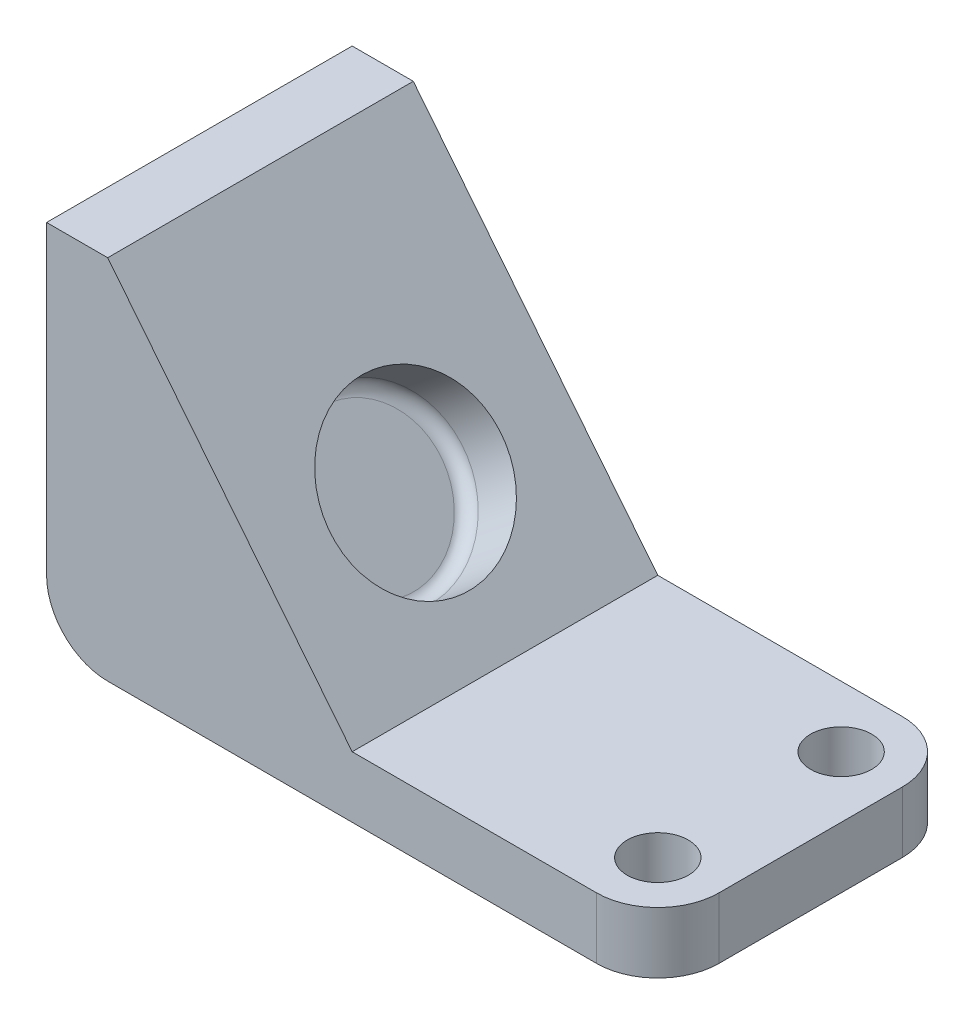
ISO-10303-21;
HEADER;
FILE_DESCRIPTION(('STEP AP214'),'2;1');
FILE_NAME('part.step','',(''),(''),'','','');
FILE_SCHEMA(('AUTOMOTIVE_DESIGN { 1 0 10303 214 1 1 1 1 }'));
ENDSEC;
DATA;
#1=APPLICATION_CONTEXT('core data for automotive mechanical design processes');
#2=APPLICATION_PROTOCOL_DEFINITION('international standard','automotive_design',2000,#1);
#3=PRODUCT_CONTEXT('',#1,'mechanical');
#4=PRODUCT('Part','Part','',(#3));
#5=PRODUCT_RELATED_PRODUCT_CATEGORY('part','',(#4));
#6=PRODUCT_DEFINITION_FORMATION('','',#4);
#7=PRODUCT_DEFINITION_CONTEXT('part definition',#1,'design');
#8=PRODUCT_DEFINITION('design','',#6,#7);
#9=PRODUCT_DEFINITION_SHAPE('','',#8);
#10=(LENGTH_UNIT() NAMED_UNIT(*) SI_UNIT(.MILLI.,.METRE.));
#11=(NAMED_UNIT(*) PLANE_ANGLE_UNIT() SI_UNIT($,.RADIAN.));
#12=(NAMED_UNIT(*) SI_UNIT($,.STERADIAN.) SOLID_ANGLE_UNIT());
#13=UNCERTAINTY_MEASURE_WITH_UNIT(LENGTH_MEASURE(1.E-05),#10,'distance_accuracy_value','');
#14=(GEOMETRIC_REPRESENTATION_CONTEXT(3) GLOBAL_UNCERTAINTY_ASSIGNED_CONTEXT((#13)) GLOBAL_UNIT_ASSIGNED_CONTEXT((#10,
#11,#12)) REPRESENTATION_CONTEXT('',''));
#15=CARTESIAN_POINT('',(0.,0.,0.));
#16=DIRECTION('',(0.,0.,1.));
#17=DIRECTION('',(1.,0.,0.));
#18=AXIS2_PLACEMENT_3D('',#15,#16,#17);
#19=CARTESIAN_POINT('',(0.,6.,2.5));
#20=DIRECTION('',(0.,-1.,0.));
#21=DIRECTION('',(0.,0.,-1.));
#22=AXIS2_PLACEMENT_3D('',#19,#20,#21);
#23=PLANE('',#22);
#24=DIRECTION('',(-1.,0.,0.));
#25=VECTOR('',#24,1.);
#26=CARTESIAN_POINT('',(0.,6.,-2.5));
#27=LINE('',#26,#25);
#28=CARTESIAN_POINT('',(1.,6.,-2.5));
#29=VERTEX_POINT('',#28);
#30=CARTESIAN_POINT('',(0.,6.,-2.5));
#31=VERTEX_POINT('',#30);
#32=EDGE_CURVE('E140',#29,#31,#27,.T.);
#33=ORIENTED_EDGE('',*,*,#32,.T.);
#34=DIRECTION('',(0.,0.,-1.));
#35=VECTOR('',#34,1.);
#36=CARTESIAN_POINT('',(0.,6.,2.5));
#37=LINE('',#36,#35);
#38=CARTESIAN_POINT('',(0.,6.,2.5));
#39=VERTEX_POINT('',#38);
#40=EDGE_CURVE('E120',#39,#31,#37,.T.);
#41=ORIENTED_EDGE('',*,*,#40,.F.);
#42=DIRECTION('',(-1.,0.,0.));
#43=VECTOR('',#42,1.);
#44=CARTESIAN_POINT('',(0.,6.,2.5));
#45=LINE('',#44,#43);
#46=CARTESIAN_POINT('',(1.,6.,2.5));
#47=VERTEX_POINT('',#46);
#48=EDGE_CURVE('E122',#47,#39,#45,.T.);
#49=ORIENTED_EDGE('',*,*,#48,.F.);
#50=DIRECTION('',(0.,0.,-1.));
#51=VECTOR('',#50,1.);
#52=CARTESIAN_POINT('',(1.,6.,2.5));
#53=LINE('',#52,#51);
#54=EDGE_CURVE('E208',#47,#29,#53,.T.);
#55=ORIENTED_EDGE('',*,*,#54,.T.);
#56=EDGE_LOOP('',(#33,#41,#49,#55));
#57=FACE_BOUND('',#56,.T.);
#58=ADVANCED_FACE('F39',(#57),#23,.F.);
#59=CARTESIAN_POINT('',(0.,1.00000000000001,2.5));
#60=DIRECTION('',(1.,0.,0.));
#61=DIRECTION('',(0.,0.,-1.));
#62=AXIS2_PLACEMENT_3D('',#59,#60,#61);
#63=PLANE('',#62);
#64=DIRECTION('',(0.,-1.,0.));
#65=VECTOR('',#64,1.);
#66=CARTESIAN_POINT('',(0.,1.00000000000001,-2.5));
#67=LINE('',#66,#65);
#68=CARTESIAN_POINT('',(0.,1.00000000000001,-2.5));
#69=VERTEX_POINT('',#68);
#70=EDGE_CURVE('E209',#31,#69,#67,.T.);
#71=ORIENTED_EDGE('',*,*,#70,.T.);
#72=DIRECTION('',(0.,0.,-1.));
#73=VECTOR('',#72,1.);
#74=CARTESIAN_POINT('',(0.,1.00000000000001,2.5));
#75=LINE('',#74,#73);
#76=CARTESIAN_POINT('',(0.,1.00000000000001,2.5));
#77=VERTEX_POINT('',#76);
#78=EDGE_CURVE('E119',#77,#69,#75,.T.);
#79=ORIENTED_EDGE('',*,*,#78,.F.);
#80=DIRECTION('',(0.,-1.,0.));
#81=VECTOR('',#80,1.);
#82=CARTESIAN_POINT('',(0.,1.00000000000001,2.5));
#83=LINE('',#82,#81);
#84=EDGE_CURVE('E114',#39,#77,#83,.T.);
#85=ORIENTED_EDGE('',*,*,#84,.F.);
#86=ORIENTED_EDGE('',*,*,#40,.T.);
#87=EDGE_LOOP('',(#71,#79,#85,#86));
#88=FACE_BOUND('',#87,.T.);
#89=ADVANCED_FACE('F113',(#88),#63,.F.);
#90=CARTESIAN_POINT('',(1.,1.,2.5));
#91=DIRECTION('',(0.,0.,-1.));
#92=DIRECTION('',(-1.,0.,0.));
#93=AXIS2_PLACEMENT_3D('',#90,#91,#92);
#94=CYLINDRICAL_SURFACE('',#93,1.);
#95=CARTESIAN_POINT('',(1.,1.,-2.5));
#96=DIRECTION('',(0.,0.,1.));
#97=DIRECTION('',(1.,0.,0.));
#98=AXIS2_PLACEMENT_3D('',#95,#96,#97);
#99=CIRCLE('',#98,1.);
#100=CARTESIAN_POINT('',(1.00000000000001,0.,-2.5));
#101=VERTEX_POINT('',#100);
#102=EDGE_CURVE('E213',#69,#101,#99,.T.);
#103=ORIENTED_EDGE('',*,*,#102,.T.);
#104=DIRECTION('',(0.,0.,-1.));
#105=VECTOR('',#104,1.);
#106=CARTESIAN_POINT('',(1.00000000000001,0.,2.5));
#107=LINE('',#106,#105);
#108=CARTESIAN_POINT('',(1.00000000000001,0.,2.5));
#109=VERTEX_POINT('',#108);
#110=EDGE_CURVE('E141',#109,#101,#107,.T.);
#111=ORIENTED_EDGE('',*,*,#110,.F.);
#112=CARTESIAN_POINT('',(1.,1.,2.5));
#113=DIRECTION('',(0.,0.,1.));
#114=DIRECTION('',(1.,0.,0.));
#115=AXIS2_PLACEMENT_3D('',#112,#113,#114);
#116=CIRCLE('',#115,1.);
#117=EDGE_CURVE('E121',#77,#109,#116,.T.);
#118=ORIENTED_EDGE('',*,*,#117,.F.);
#119=ORIENTED_EDGE('',*,*,#78,.T.);
#120=EDGE_LOOP('',(#103,#111,#118,#119));
#121=FACE_BOUND('',#120,.T.);
#122=ADVANCED_FACE('F176',(#121),#94,.T.);
#123=CARTESIAN_POINT('',(10.,0.,2.5));
#124=DIRECTION('',(0.,1.,0.));
#125=DIRECTION('',(-1.,0.,0.));
#126=AXIS2_PLACEMENT_3D('',#123,#124,#125);
#127=PLANE('',#126);
#128=CARTESIAN_POINT('',(9.,0.,1.5));
#129=DIRECTION('',(0.,1.,0.));
#130=DIRECTION('',(0.,0.,1.));
#131=AXIS2_PLACEMENT_3D('',#128,#129,#130);
#132=CIRCLE('',#131,0.500000000000001);
#133=CARTESIAN_POINT('',(9.,0.,2.));
#134=VERTEX_POINT('',#133);
#135=EDGE_CURVE('E275',#134,#134,#132,.T.);
#136=ORIENTED_EDGE('',*,*,#135,.T.);
#137=EDGE_LOOP('',(#136));
#138=FACE_BOUND('',#137,.T.);
#139=CARTESIAN_POINT('',(9.,0.,-1.5));
#140=DIRECTION('',(0.,1.,0.));
#141=DIRECTION('',(0.,0.,1.));
#142=AXIS2_PLACEMENT_3D('',#139,#140,#141);
#143=CIRCLE('',#142,0.500000000000001);
#144=CARTESIAN_POINT('',(9.,0.,-0.999999999999999));
#145=VERTEX_POINT('',#144);
#146=EDGE_CURVE('E262',#145,#145,#143,.T.);
#147=ORIENTED_EDGE('',*,*,#146,.T.);
#148=EDGE_LOOP('',(#147));
#149=FACE_BOUND('',#148,.T.);
#150=DIRECTION('',(0.,0.,-1.));
#151=VECTOR('',#150,1.);
#152=CARTESIAN_POINT('',(10.,0.,2.5));
#153=LINE('',#152,#151);
#154=CARTESIAN_POINT('',(10.,0.,1.5));
#155=VERTEX_POINT('',#154);
#156=CARTESIAN_POINT('',(10.,0.,-1.5));
#157=VERTEX_POINT('',#156);
#158=EDGE_CURVE('E200',#155,#157,#153,.T.);
#159=ORIENTED_EDGE('',*,*,#158,.F.);
#160=CARTESIAN_POINT('',(9.,0.,1.5));
#161=DIRECTION('',(0.,1.,0.));
#162=DIRECTION('',(-1.,0.,0.));
#163=AXIS2_PLACEMENT_3D('',#160,#161,#162);
#164=CIRCLE('',#163,1.);
#165=CARTESIAN_POINT('',(9.,0.,2.5));
#166=VERTEX_POINT('',#165);
#167=EDGE_CURVE('E156',#155,#166,#164,.F.);
#168=ORIENTED_EDGE('',*,*,#167,.T.);
#169=DIRECTION('',(1.,0.,0.));
#170=VECTOR('',#169,1.);
#171=CARTESIAN_POINT('',(10.,0.,2.5));
#172=LINE('',#171,#170);
#173=EDGE_CURVE('E196',#109,#166,#172,.T.);
#174=ORIENTED_EDGE('',*,*,#173,.F.);
#175=ORIENTED_EDGE('',*,*,#110,.T.);
#176=DIRECTION('',(1.,0.,0.));
#177=VECTOR('',#176,1.);
#178=CARTESIAN_POINT('',(10.,0.,-2.5));
#179=LINE('',#178,#177);
#180=CARTESIAN_POINT('',(9.,0.,-2.5));
#181=VERTEX_POINT('',#180);
#182=EDGE_CURVE('E214',#101,#181,#179,.T.);
#183=ORIENTED_EDGE('',*,*,#182,.T.);
#184=CARTESIAN_POINT('',(9.,0.,-1.5));
#185=DIRECTION('',(0.,1.,0.));
#186=DIRECTION('',(-1.,0.,0.));
#187=AXIS2_PLACEMENT_3D('',#184,#185,#186);
#188=CIRCLE('',#187,1.);
#189=EDGE_CURVE('E61',#181,#157,#188,.F.);
#190=ORIENTED_EDGE('',*,*,#189,.T.);
#191=EDGE_LOOP('',(#159,#168,#174,#175,#183,#190));
#192=FACE_BOUND('',#191,.T.);
#193=ADVANCED_FACE('F198',(#138,#149,#192),#127,.F.);
#194=CARTESIAN_POINT('',(10.,0.999999999999999,2.5));
#195=DIRECTION('',(-1.,0.,0.));
#196=DIRECTION('',(0.,0.,1.));
#197=AXIS2_PLACEMENT_3D('',#194,#195,#196);
#198=PLANE('',#197);
#199=DIRECTION('',(0.,0.,-1.));
#200=VECTOR('',#199,1.);
#201=CARTESIAN_POINT('',(10.,0.999999999999999,2.5));
#202=LINE('',#201,#200);
#203=CARTESIAN_POINT('',(10.,0.999999999999999,1.5));
#204=VERTEX_POINT('',#203);
#205=CARTESIAN_POINT('',(10.,0.999999999999999,-1.5));
#206=VERTEX_POINT('',#205);
#207=EDGE_CURVE('E221',#204,#206,#202,.T.);
#208=ORIENTED_EDGE('',*,*,#207,.F.);
#209=DIRECTION('',(0.,1.,0.));
#210=VECTOR('',#209,1.);
#211=CARTESIAN_POINT('',(10.,0.,1.5));
#212=LINE('',#211,#210);
#213=EDGE_CURVE('E153',#204,#155,#212,.F.);
#214=ORIENTED_EDGE('',*,*,#213,.T.);
#215=ORIENTED_EDGE('',*,*,#158,.T.);
#216=DIRECTION('',(0.,1.,0.));
#217=VECTOR('',#216,1.);
#218=CARTESIAN_POINT('',(10.,0.999999999999999,-1.5));
#219=LINE('',#218,#217);
#220=EDGE_CURVE('E147',#157,#206,#219,.T.);
#221=ORIENTED_EDGE('',*,*,#220,.T.);
#222=EDGE_LOOP('',(#208,#214,#215,#221));
#223=FACE_BOUND('',#222,.T.);
#224=ADVANCED_FACE('F234',(#223),#198,.F.);
#225=CARTESIAN_POINT('',(5.,0.999999999999999,2.5));
#226=DIRECTION('',(0.,-1.,0.));
#227=DIRECTION('',(0.,0.,-1.));
#228=AXIS2_PLACEMENT_3D('',#225,#226,#227);
#229=PLANE('',#228);
#230=CARTESIAN_POINT('',(9.,0.999999999999999,1.5));
#231=DIRECTION('',(0.,1.,0.));
#232=DIRECTION('',(0.,0.,1.));
#233=AXIS2_PLACEMENT_3D('',#230,#231,#232);
#234=CIRCLE('',#233,0.500000000000001);
#235=CARTESIAN_POINT('',(9.,0.999999999999999,2.));
#236=VERTEX_POINT('',#235);
#237=EDGE_CURVE('E267',#236,#236,#234,.T.);
#238=ORIENTED_EDGE('',*,*,#237,.F.);
#239=EDGE_LOOP('',(#238));
#240=FACE_BOUND('',#239,.T.);
#241=CARTESIAN_POINT('',(9.,0.999999999999999,-1.5));
#242=DIRECTION('',(0.,1.,0.));
#243=DIRECTION('',(0.,0.,1.));
#244=AXIS2_PLACEMENT_3D('',#241,#242,#243);
#245=CIRCLE('',#244,0.500000000000001);
#246=CARTESIAN_POINT('',(9.,0.999999999999999,-0.999999999999999));
#247=VERTEX_POINT('',#246);
#248=EDGE_CURVE('E270',#247,#247,#245,.T.);
#249=ORIENTED_EDGE('',*,*,#248,.F.);
#250=EDGE_LOOP('',(#249));
#251=FACE_BOUND('',#250,.T.);
#252=DIRECTION('',(-1.,0.,0.));
#253=VECTOR('',#252,1.);
#254=CARTESIAN_POINT('',(5.,0.999999999999999,2.5));
#255=LINE('',#254,#253);
#256=CARTESIAN_POINT('',(9.,0.999999999999999,2.5));
#257=VERTEX_POINT('',#256);
#258=CARTESIAN_POINT('',(5.,0.999999999999999,2.5));
#259=VERTEX_POINT('',#258);
#260=EDGE_CURVE('E205',#257,#259,#255,.T.);
#261=ORIENTED_EDGE('',*,*,#260,.F.);
#262=CARTESIAN_POINT('',(9.,0.999999999999999,1.5));
#263=DIRECTION('',(0.,-1.,0.));
#264=DIRECTION('',(0.,0.,-1.));
#265=AXIS2_PLACEMENT_3D('',#262,#263,#264);
#266=CIRCLE('',#265,1.);
#267=EDGE_CURVE('E146',#257,#204,#266,.F.);
#268=ORIENTED_EDGE('',*,*,#267,.T.);
#269=ORIENTED_EDGE('',*,*,#207,.T.);
#270=CARTESIAN_POINT('',(9.,0.999999999999999,-1.5));
#271=DIRECTION('',(0.,-1.,0.));
#272=DIRECTION('',(0.,0.,-1.));
#273=AXIS2_PLACEMENT_3D('',#270,#271,#272);
#274=CIRCLE('',#273,1.);
#275=CARTESIAN_POINT('',(9.,0.999999999999999,-2.5));
#276=VERTEX_POINT('',#275);
#277=EDGE_CURVE('E143',#206,#276,#274,.F.);
#278=ORIENTED_EDGE('',*,*,#277,.T.);
#279=DIRECTION('',(-1.,0.,0.));
#280=VECTOR('',#279,1.);
#281=CARTESIAN_POINT('',(5.,0.999999999999999,-2.5));
#282=LINE('',#281,#280);
#283=CARTESIAN_POINT('',(5.,0.999999999999999,-2.5));
#284=VERTEX_POINT('',#283);
#285=EDGE_CURVE('E220',#276,#284,#282,.T.);
#286=ORIENTED_EDGE('',*,*,#285,.T.);
#287=DIRECTION('',(0.,0.,-1.));
#288=VECTOR('',#287,1.);
#289=CARTESIAN_POINT('',(5.,0.999999999999999,2.5));
#290=LINE('',#289,#288);
#291=EDGE_CURVE('E222',#259,#284,#290,.T.);
#292=ORIENTED_EDGE('',*,*,#291,.F.);
#293=EDGE_LOOP('',(#261,#268,#269,#278,#286,#292));
#294=FACE_BOUND('',#293,.T.);
#295=ADVANCED_FACE('F241',(#240,#251,#294),#229,.F.);
#296=CARTESIAN_POINT('',(1.,6.,2.5));
#297=DIRECTION('',(-0.78086880944303,-0.624695047554424,0.));
#298=DIRECTION('',(0.624695047554424,-0.78086880944303,0.));
#299=AXIS2_PLACEMENT_3D('',#296,#297,#298);
#300=PLANE('',#299);
#301=CARTESIAN_POINT('',(3.53658536585366,2.82926829268293,0.));
#302=DIRECTION('',(0.78086880944303,0.624695047554424,0.));
#303=DIRECTION('',(-0.624695047554424,0.78086880944303,0.));
#304=AXIS2_PLACEMENT_3D('',#301,#302,#303);
#305=CIRCLE('',#304,1.4);
#306=CARTESIAN_POINT('',(2.66201229927746,3.92248462590317,0.));
#307=VERTEX_POINT('',#306);
#308=EDGE_CURVE('E211',#307,#307,#305,.T.);
#309=ORIENTED_EDGE('',*,*,#308,.F.);
#310=EDGE_LOOP('',(#309));
#311=FACE_BOUND('',#310,.T.);
#312=DIRECTION('',(-0.624695047554424,0.78086880944303,0.));
#313=VECTOR('',#312,1.);
#314=CARTESIAN_POINT('',(1.,6.,-2.5));
#315=LINE('',#314,#313);
#316=EDGE_CURVE('E133',#284,#29,#315,.T.);
#317=ORIENTED_EDGE('',*,*,#316,.T.);
#318=ORIENTED_EDGE('',*,*,#54,.F.);
#319=DIRECTION('',(-0.624695047554424,0.78086880944303,0.));
#320=VECTOR('',#319,1.);
#321=CARTESIAN_POINT('',(1.,6.,2.5));
#322=LINE('',#321,#320);
#323=EDGE_CURVE('E128',#259,#47,#322,.T.);
#324=ORIENTED_EDGE('',*,*,#323,.F.);
#325=ORIENTED_EDGE('',*,*,#291,.T.);
#326=EDGE_LOOP('',(#317,#318,#324,#325));
#327=FACE_BOUND('',#326,.T.);
#328=ADVANCED_FACE('F244',(#311,#327),#300,.F.);
#329=CARTESIAN_POINT('',(1.,1.,2.5));
#330=DIRECTION('',(0.,0.,1.));
#331=DIRECTION('',(1.,0.,0.));
#332=AXIS2_PLACEMENT_3D('',#329,#330,#331);
#333=PLANE('',#332);
#334=ORIENTED_EDGE('',*,*,#173,.T.);
#335=DIRECTION('',(0.,1.,0.));
#336=VECTOR('',#335,1.);
#337=CARTESIAN_POINT('',(9.,0.999999999999999,2.5));
#338=LINE('',#337,#336);
#339=EDGE_CURVE('E136',#166,#257,#338,.T.);
#340=ORIENTED_EDGE('',*,*,#339,.T.);
#341=ORIENTED_EDGE('',*,*,#260,.T.);
#342=ORIENTED_EDGE('',*,*,#323,.T.);
#343=ORIENTED_EDGE('',*,*,#48,.T.);
#344=ORIENTED_EDGE('',*,*,#84,.T.);
#345=ORIENTED_EDGE('',*,*,#117,.T.);
#346=EDGE_LOOP('',(#334,#340,#341,#342,#343,#344,#345));
#347=FACE_BOUND('',#346,.T.);
#348=ADVANCED_FACE('F126',(#347),#333,.T.);
#349=CARTESIAN_POINT('',(1.,1.,-2.5));
#350=DIRECTION('',(0.,0.,1.));
#351=DIRECTION('',(1.,0.,0.));
#352=AXIS2_PLACEMENT_3D('',#349,#350,#351);
#353=PLANE('',#352);
#354=ORIENTED_EDGE('',*,*,#285,.F.);
#355=DIRECTION('',(0.,1.,0.));
#356=VECTOR('',#355,1.);
#357=CARTESIAN_POINT('',(9.,1.,-2.5));
#358=LINE('',#357,#356);
#359=EDGE_CURVE('E53',#276,#181,#358,.F.);
#360=ORIENTED_EDGE('',*,*,#359,.T.);
#361=ORIENTED_EDGE('',*,*,#182,.F.);
#362=ORIENTED_EDGE('',*,*,#102,.F.);
#363=ORIENTED_EDGE('',*,*,#70,.F.);
#364=ORIENTED_EDGE('',*,*,#32,.F.);
#365=ORIENTED_EDGE('',*,*,#316,.F.);
#366=EDGE_LOOP('',(#354,#360,#361,#362,#363,#364,#365));
#367=FACE_BOUND('',#366,.T.);
#368=ADVANCED_FACE('F228',(#367),#353,.F.);
#369=CARTESIAN_POINT('',(2.75571655641063,2.2045732451285,0.));
#370=DIRECTION('',(0.78086880944303,0.624695047554424,0.));
#371=DIRECTION('',(-0.624695047554424,0.78086880944303,0.));
#372=AXIS2_PLACEMENT_3D('',#369,#370,#371);
#373=CYLINDRICAL_SURFACE('',#372,1.4);
#374=CARTESIAN_POINT('',(2.91189031829923,2.32951225463939,0.));
#375=DIRECTION('',(0.78086880944303,0.624695047554424,0.));
#376=DIRECTION('',(-0.624695047554424,0.78086880944303,0.));
#377=AXIS2_PLACEMENT_3D('',#374,#375,#376);
#378=CIRCLE('',#377,1.4);
#379=CARTESIAN_POINT('',(2.03731725172304,3.42272858785963,0.));
#380=VERTEX_POINT('',#379);
#381=EDGE_CURVE('E11',#380,#380,#378,.F.);
#382=ORIENTED_EDGE('',*,*,#381,.T.);
#383=EDGE_LOOP('',(#382));
#384=FACE_BOUND('',#383,.T.);
#385=ORIENTED_EDGE('',*,*,#308,.T.);
#386=EDGE_LOOP('',(#385));
#387=FACE_BOUND('',#386,.T.);
#388=ADVANCED_FACE('F249',(#384,#387),#373,.F.);
#389=CARTESIAN_POINT('',(2.75571655641063,2.2045732451285,0.));
#390=DIRECTION('',(0.78086880944303,0.624695047554424,0.));
#391=DIRECTION('',(-0.624695047554424,0.78086880944303,0.));
#392=AXIS2_PLACEMENT_3D('',#389,#390,#391);
#393=PLANE('',#392);
#394=CARTESIAN_POINT('',(2.75571655641063,2.2045732451285,0.));
#395=DIRECTION('',(0.78086880944303,0.624695047554424,0.));
#396=DIRECTION('',(-0.624695047554424,0.78086880944303,0.));
#397=AXIS2_PLACEMENT_3D('',#394,#395,#396);
#398=CIRCLE('',#397,1.2);
#399=CARTESIAN_POINT('',(2.00608249934532,3.14161581646014,0.));
#400=VERTEX_POINT('',#399);
#401=EDGE_CURVE('E50',#400,#400,#398,.T.);
#402=ORIENTED_EDGE('',*,*,#401,.T.);
#403=EDGE_LOOP('',(#402));
#404=FACE_BOUND('',#403,.T.);
#405=ADVANCED_FACE('F161',(#404),#393,.T.);
#406=CARTESIAN_POINT('',(9.,0.,-1.5));
#407=DIRECTION('',(0.,1.,0.));
#408=DIRECTION('',(0.,0.,1.));
#409=AXIS2_PLACEMENT_3D('',#406,#407,#408);
#410=CYLINDRICAL_SURFACE('',#409,0.500000000000001);
#411=ORIENTED_EDGE('',*,*,#146,.F.);
#412=EDGE_LOOP('',(#411));
#413=FACE_BOUND('',#412,.T.);
#414=ORIENTED_EDGE('',*,*,#248,.T.);
#415=EDGE_LOOP('',(#414));
#416=FACE_BOUND('',#415,.T.);
#417=ADVANCED_FACE('F188',(#413,#416),#410,.F.);
#418=CARTESIAN_POINT('',(9.,0.,1.5));
#419=DIRECTION('',(0.,1.,0.));
#420=DIRECTION('',(0.,0.,1.));
#421=AXIS2_PLACEMENT_3D('',#418,#419,#420);
#422=CYLINDRICAL_SURFACE('',#421,0.500000000000001);
#423=ORIENTED_EDGE('',*,*,#135,.F.);
#424=EDGE_LOOP('',(#423));
#425=FACE_BOUND('',#424,.T.);
#426=ORIENTED_EDGE('',*,*,#237,.T.);
#427=EDGE_LOOP('',(#426));
#428=FACE_BOUND('',#427,.T.);
#429=ADVANCED_FACE('F181',(#425,#428),#422,.F.);
#430=CARTESIAN_POINT('',(9.,1.,1.5));
#431=DIRECTION('',(0.,-1.,0.));
#432=DIRECTION('',(0.,0.,-1.));
#433=AXIS2_PLACEMENT_3D('',#430,#431,#432);
#434=CYLINDRICAL_SURFACE('',#433,1.);
#435=ORIENTED_EDGE('',*,*,#167,.F.);
#436=ORIENTED_EDGE('',*,*,#213,.F.);
#437=ORIENTED_EDGE('',*,*,#267,.F.);
#438=ORIENTED_EDGE('',*,*,#339,.F.);
#439=EDGE_LOOP('',(#435,#436,#437,#438));
#440=FACE_BOUND('',#439,.T.);
#441=ADVANCED_FACE('F168',(#440),#434,.T.);
#442=CARTESIAN_POINT('',(9.,0.999999999999999,-1.5));
#443=DIRECTION('',(0.,1.,0.));
#444=DIRECTION('',(0.,0.,1.));
#445=AXIS2_PLACEMENT_3D('',#442,#443,#444);
#446=CYLINDRICAL_SURFACE('',#445,1.);
#447=ORIENTED_EDGE('',*,*,#189,.F.);
#448=ORIENTED_EDGE('',*,*,#359,.F.);
#449=ORIENTED_EDGE('',*,*,#277,.F.);
#450=ORIENTED_EDGE('',*,*,#220,.F.);
#451=EDGE_LOOP('',(#447,#448,#449,#450));
#452=FACE_BOUND('',#451,.T.);
#453=ADVANCED_FACE('F163',(#452),#446,.T.);
#454=CARTESIAN_POINT('',(2.91189031829923,2.32951225463939,0.));
#455=DIRECTION('',(0.78086880944303,0.624695047554424,0.));
#456=DIRECTION('',(-0.624695047554424,0.78086880944303,0.));
#457=AXIS2_PLACEMENT_3D('',#454,#455,#456);
#458=TOROIDAL_SURFACE('',#457,1.2,0.2);
#459=ORIENTED_EDGE('',*,*,#381,.F.);
#460=EDGE_LOOP('',(#459));
#461=FACE_BOUND('',#460,.T.);
#462=ORIENTED_EDGE('',*,*,#401,.F.);
#463=EDGE_LOOP('',(#462));
#464=FACE_BOUND('',#463,.T.);
#465=ADVANCED_FACE('F41',(#461,#464),#458,.F.);
#466=CLOSED_SHELL('',(#58,#89,#122,#193,#224,#295,#328,#348,#368,#388,#405,#417,#429,#441,#453,#465));
#467=MANIFOLD_SOLID_BREP('B2',#466);
#468=ADVANCED_BREP_SHAPE_REPRESENTATION('',(#18,#467),#14);
#469=SHAPE_DEFINITION_REPRESENTATION(#9,#468);
ENDSEC;
END-ISO-10303-21;
